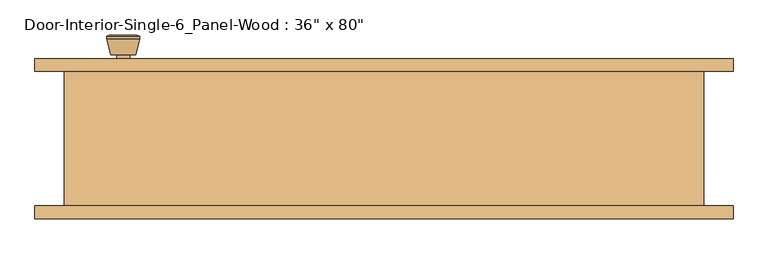
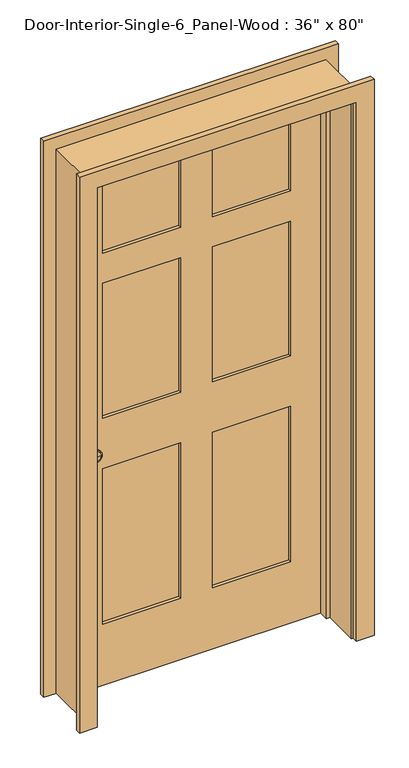
"""IFC4 building model written with IfcOpenShell, lengths in millimetres: door geometry."""

from ifc_helpers import new_model, si_unit, point, frame, frame_2d, origin, place, context, project, spatial, polyline, circle_curve, trimmed, segment, composite_curve, outline, extrude, faceted_brep, source, transform, mapped, element, save
from ifc_brep_helpers import plane_surface, cylinder_surface, revolved_surface, advanced_brep


def door_5dfbd760(model_context):
    return source(origin(), model_context, "Body", "SolidModel", [
        advanced_brep(
        [(-393.7, 57.5, 914.4), (-383.7, 57.5, 914.4), (-403.7, 57.5, 914.4), (-373.2241324, 8.5, 914.4), (-393.7, 8.5, 914.4), (-414.1758676, 8.5, 914.4), (-368.7, 10.3278681, 914.4), (-418.7, 10.3278681, 914.4), (-368.7, 13.7915463, 914.4), (-418.7, 13.7915463, 914.4), (-375.063764, 38.5, 914.4), (-412.336236, 38.5, 914.4), (-383.7, 38.5, 914.4), (-403.7, 38.5, 914.4)],
        [
            (0, 1),
            (1, 2, circle_curve(frame((-393.7, 57.5, 914.4), z_axis=(0.0, 1.0, 0.0), x_axis=(-1.0, 0.0, 0.0)), 10.0)),
            (2, 0),
            (2, 1, circle_curve(frame((-393.7, 57.5, 914.4), z_axis=(0.0, 1.0, 0.0), x_axis=(-1.0, 0.0, 0.0)), 10.0)),
            (3, 4),
            (4, 5),
            (5, 3, circle_curve(frame((-393.7, 8.5, 914.4), z_axis=(0.0, -1.0, 0.0), x_axis=(-1.0, 0.0, 0.0)), 20.4758676)),
            (3, 5, circle_curve(frame((-393.7, 8.5, 914.4), z_axis=(0.0, -1.0, 0.0), x_axis=(-1.0, 0.0, 0.0)), 20.4758676)),
            (6, 3),
            (5, 7),
            (7, 6, circle_curve(frame((-393.7, 10.3278681, 914.4), z_axis=(0.0, -1.0, 0.0), x_axis=(-1.0, 0.0, 0.0)), 25.0)),
            (6, 7, circle_curve(frame((-393.7, 10.3278681, 914.4), z_axis=(0.0, -1.0, 0.0), x_axis=(-1.0, 0.0, 0.0)), 25.0)),
            (8, 6),
            (7, 9),
            (9, 8, circle_curve(frame((-393.7, 13.7915463, 914.4), z_axis=(0.0, -1.0, 0.0), x_axis=(-1.0, 0.0, 0.0)), 25.0)),
            (8, 9, circle_curve(frame((-393.7, 13.7915463, 914.4), z_axis=(0.0, -1.0, 0.0), x_axis=(-1.0, 0.0, 0.0)), 25.0)),
            (10, 8),
            (9, 11),
            (11, 10, circle_curve(frame((-393.7, 38.5, 914.4), z_axis=(0.0, -1.0, 0.0), x_axis=(-1.0, 0.0, 0.0)), 18.636236)),
            (10, 11, circle_curve(frame((-393.7, 38.5, 914.4), z_axis=(0.0, -1.0, 0.0), x_axis=(-1.0, 0.0, 0.0)), 18.636236)),
            (12, 10),
            (11, 13),
            (13, 12, circle_curve(frame((-393.7, 38.5, 914.4), z_axis=(0.0, -1.0, 0.0), x_axis=(-1.0, 0.0, 0.0)), 10.0)),
            (12, 13, circle_curve(frame((-393.7, 38.5, 914.4), z_axis=(0.0, -1.0, 0.0), x_axis=(-1.0, 0.0, 0.0)), 10.0)),
            (1, 12),
            (13, 2),
        ],
        [
            plane_surface(frame((-393.7, 57.5, 914.4), z_axis=(0.0, 1.0, 0.0), x_axis=(-1.0, 0.0, 0.0))),
            plane_surface(frame((-393.7, 8.5, 914.4), z_axis=(0.0, -1.0, 0.0), x_axis=(-1.0, 0.0, 0.0))),
            revolved_surface(polyline([(-414.1758676, 8.5, 914.4), (-418.7, 10.3278681, 914.4)]), (-393.7, 57.5, 914.4), (0.0, 1.0, 0.0)),
            cylinder_surface(frame((-393.7, 57.5, 914.4), z_axis=(0.0, 1.0, 0.0), x_axis=(-1.0, 0.0, 0.0)), 25.0),
            revolved_surface(polyline([(-418.7, 13.7915463, 914.4), (-412.336236, 38.5, 914.4)]), (-393.7, 57.5, 914.4), (0.0, 1.0, 0.0)),
            plane_surface(frame((-393.7, 38.5, 914.4), z_axis=(0.0, 1.0, 0.0), x_axis=(-1.0, 0.0, 0.0))),
            cylinder_surface(frame((-393.7, 57.5, 914.4), z_axis=(0.0, 1.0, 0.0), x_axis=(-1.0, 0.0, 0.0)), 10.0),
        ],
        [
            (0, [[1, 2, 3]]),
            (0, [[-3, 4, -1]]),
            (1, [[5, 6, 7]]),
            (1, [[-6, -5, 8]]),
            (2, [[9, -7, 10, 11]]),
            (2, [[-10, -8, -9, 12]]),
            (3, [[13, -11, 14, 15]]),
            (3, [[-14, -12, -13, 16]]),
            (4, [[17, -15, 18, 19]]),
            (4, [[-18, -16, -17, 20]]),
            (5, [[21, -19, 22, 23]]),
            (5, [[-22, -20, -21, 24]]),
            (6, [[25, -23, 26, -2]]),
            (6, [[-26, -24, -25, -4]]),
        ],
    ),
        extrude(outline(composite_curve([segment(trimmed(circle_curve(frame_2d((914.4, -393.7)), 30.0), [point((914.4, -423.7))], [point((914.4, -363.7))], False, "CARTESIAN"), True, "CONTINUOUS"), segment(trimmed(circle_curve(frame_2d((914.4, -393.7)), 30.0), [point((914.4, -363.7))], [point((914.4, -423.7))], False, "CARTESIAN"), True, "CONTINUOUS")], self_intersect=False)), frame((0.0, 57.5, 0.0), z_axis=(0.0, 1.0, 0.0), x_axis=(0.0, 0.0, 1.0)), (0.0, 0.0, 1.0), 6.0),
        advanced_brep(
        [(-393.7, 104.425, 914.4), (-403.7, 104.425, 914.4), (-383.7, 104.425, 914.4), (-373.2241324, 153.425, 914.4), (-414.1758676, 153.425, 914.4), (-393.7, 153.425, 914.4), (-368.7, 151.5971319, 914.4), (-418.7, 151.5971319, 914.4), (-368.7, 148.1334537, 914.4), (-418.7, 148.1334537, 914.4), (-375.063764, 123.425, 914.4), (-412.336236, 123.425, 914.4), (-383.7, 123.425, 914.4), (-403.7, 123.425, 914.4)],
        [
            (0, 1),
            (1, 2, circle_curve(frame((-393.7, 104.425, 914.4), z_axis=(0.0, -1.0, 0.0), x_axis=(-1.0, 0.0, 0.0)), 10.0)),
            (2, 0),
            (2, 1, circle_curve(frame((-393.7, 104.425, 914.4), z_axis=(0.0, -1.0, 0.0), x_axis=(-1.0, 0.0, 0.0)), 10.0)),
            (3, 4, circle_curve(frame((-393.7, 153.425, 914.4), z_axis=(0.0, 1.0, 0.0), x_axis=(-1.0, 0.0, 0.0)), 20.4758676)),
            (4, 5),
            (5, 3),
            (4, 3, circle_curve(frame((-393.7, 153.425, 914.4), z_axis=(0.0, 1.0, 0.0), x_axis=(-1.0, 0.0, 0.0)), 20.4758676)),
            (6, 7, circle_curve(frame((-393.7, 151.5971319, 914.4), z_axis=(0.0, 1.0, 0.0), x_axis=(-1.0, 0.0, 0.0)), 25.0)),
            (7, 4),
            (3, 6),
            (7, 6, circle_curve(frame((-393.7, 151.5971319, 914.4), z_axis=(0.0, 1.0, 0.0), x_axis=(-1.0, 0.0, 0.0)), 25.0)),
            (8, 9, circle_curve(frame((-393.7, 148.1334537, 914.4), z_axis=(0.0, 1.0, 0.0), x_axis=(-1.0, 0.0, 0.0)), 25.0)),
            (9, 7),
            (6, 8),
            (9, 8, circle_curve(frame((-393.7, 148.1334537, 914.4), z_axis=(0.0, 1.0, 0.0), x_axis=(-1.0, 0.0, 0.0)), 25.0)),
            (10, 11, circle_curve(frame((-393.7, 123.425, 914.4), z_axis=(0.0, 1.0, 0.0), x_axis=(-1.0, 0.0, 0.0)), 18.636236)),
            (11, 9),
            (8, 10),
            (11, 10, circle_curve(frame((-393.7, 123.425, 914.4), z_axis=(0.0, 1.0, 0.0), x_axis=(-1.0, 0.0, 0.0)), 18.636236)),
            (12, 13, circle_curve(frame((-393.7, 123.425, 914.4), z_axis=(0.0, 1.0, 0.0), x_axis=(-1.0, 0.0, 0.0)), 10.0)),
            (13, 11),
            (10, 12),
            (13, 12, circle_curve(frame((-393.7, 123.425, 914.4), z_axis=(0.0, 1.0, 0.0), x_axis=(-1.0, 0.0, 0.0)), 10.0)),
            (1, 13),
            (12, 2),
        ],
        [
            plane_surface(frame((-393.7, 104.425, 914.4), z_axis=(0.0, -1.0, 0.0), x_axis=(-1.0, 0.0, 0.0))),
            plane_surface(frame((-393.7, 153.425, 914.4), z_axis=(0.0, 1.0, 0.0), x_axis=(-1.0, 0.0, 0.0))),
            revolved_surface(polyline([(-414.1758676, 153.425, 914.4), (-418.7, 151.5971319, 914.4)]), (-393.7, 104.425, 914.4), (0.0, -1.0, 0.0)),
            cylinder_surface(frame((-393.7, 104.425, 914.4), z_axis=(0.0, -1.0, 0.0), x_axis=(-1.0, 0.0, 0.0)), 25.0),
            revolved_surface(polyline([(-418.7, 148.1334537, 914.4), (-412.336236, 123.425, 914.4)]), (-393.7, 104.425, 914.4), (0.0, -1.0, 0.0)),
            plane_surface(frame((-393.7, 123.425, 914.4), z_axis=(0.0, -1.0, 0.0), x_axis=(-1.0, 0.0, 0.0))),
            cylinder_surface(frame((-393.7, 104.425, 914.4), z_axis=(0.0, -1.0, 0.0), x_axis=(-1.0, 0.0, 0.0)), 10.0),
        ],
        [
            (0, [[1, 2, 3]]),
            (0, [[-3, 4, -1]]),
            (1, [[5, 6, 7]]),
            (1, [[8, -7, -6]]),
            (2, [[9, 10, -5, 11]]),
            (2, [[12, -11, -8, -10]]),
            (3, [[13, 14, -9, 15]]),
            (3, [[16, -15, -12, -14]]),
            (4, [[17, 18, -13, 19]]),
            (4, [[20, -19, -16, -18]]),
            (5, [[21, 22, -17, 23]]),
            (5, [[24, -23, -20, -22]]),
            (6, [[-2, 25, -21, 26]]),
            (6, [[-4, -26, -24, -25]]),
        ],
    ),
        extrude(outline(composite_curve([segment(trimmed(circle_curve(frame_2d((914.4, -393.7)), 30.0), [point((914.4, -423.7))], [point((914.4, -363.7))], False, "CARTESIAN"), True, "CONTINUOUS"), segment(trimmed(circle_curve(frame_2d((914.4, -393.7)), 30.0), [point((914.4, -363.7))], [point((914.4, -423.7))], False, "CARTESIAN"), True, "CONTINUOUS")], self_intersect=False)), frame((0.0, 98.425, 0.0), z_axis=(0.0, 1.0, 0.0), x_axis=(0.0, 0.0, 1.0)), (0.0, 0.0, 1.0), 6.0),
        extrude(outline(polyline([(336.55, 75.1416667), (57.15, 75.1416667), (57.15, 86.7833333), (336.55, 86.7833333), (336.55, 75.1416667)])), frame((0.0, 0.0, 1633.5375), z_axis=(0.0, 0.0, 1.0), x_axis=(1.0, 0.0, 0.0)), (0.0, 0.0, 1.0), 279.4),
        extrude(outline(polyline([(336.55, 75.1416667), (57.15, 75.1416667), (57.15, 86.7833333), (336.55, 86.7833333), (336.55, 75.1416667)])), frame((0.0, 0.0, 1009.65), z_axis=(0.0, 0.0, 1.0), x_axis=(1.0, 0.0, 0.0)), (0.0, 0.0, 1.0), 509.5875),
        extrude(outline(polyline([(-57.15, 75.1416667), (-336.55, 75.1416667), (-336.55, 86.7833333), (-57.15, 86.7833333), (-57.15, 75.1416667)])), frame((0.0, 0.0, 1009.65), z_axis=(0.0, 0.0, 1.0), x_axis=(1.0, 0.0, 0.0)), (0.0, 0.0, 1.0), 509.5875),
        extrude(outline(polyline([(-57.15, 75.1416667), (-336.55, 75.1416667), (-336.55, 86.7833333), (-57.15, 86.7833333), (-57.15, 75.1416667)])), frame((0.0, 0.0, 1633.5375), z_axis=(0.0, 0.0, 1.0), x_axis=(1.0, 0.0, 0.0)), (0.0, 0.0, 1.0), 279.4),
        extrude(outline(polyline([(336.55, 75.1416667), (57.15, 75.1416667), (57.15, 86.7833333), (336.55, 86.7833333), (336.55, 75.1416667)])), frame((0.0, 0.0, 231.775), z_axis=(0.0, 0.0, 1.0), x_axis=(1.0, 0.0, 0.0)), (0.0, 0.0, 1.0), 587.375),
        extrude(outline(polyline([(-57.15, 75.1416667), (-336.55, 75.1416667), (-336.55, 86.7833333), (-57.15, 86.7833333), (-57.15, 75.1416667)])), frame((0.0, 0.0, 231.775), z_axis=(0.0, 0.0, 1.0), x_axis=(1.0, 0.0, 0.0)), (0.0, 0.0, 1.0), 587.375),
        extrude(outline(polyline([(2032.0, -457.2), (0.0, -457.2), (0.0, 457.2), (2032.0, 457.2), (2032.0, -457.2)]), holes=[polyline([(1912.9375, 57.15), (1912.9375, 336.55), (1633.5375, 336.55), (1633.5375, 57.15), (1912.9375, 57.15)]), polyline([(1519.2375, 336.55), (1009.65, 336.55), (1009.65, 57.15), (1519.2375, 57.15), (1519.2375, 336.55)]), polyline([(1009.65, -57.15), (1009.65, -336.55), (1519.2375, -336.55), (1519.2375, -57.15), (1009.65, -57.15)]), polyline([(1633.5375, -336.55), (1912.9375, -336.55), (1912.9375, -57.15), (1633.5375, -57.15), (1633.5375, -336.55)]), polyline([(819.15, 57.15), (819.15, 336.55), (231.775, 336.55), (231.775, 57.15), (819.15, 57.15)]), polyline([(231.775, -57.15), (231.775, -336.55), (819.15, -336.55), (819.15, -57.15), (231.775, -57.15)])]), frame((0.0, 63.5, 0.0), z_axis=(0.0, 1.0, 0.0), x_axis=(0.0, 0.0, 1.0)), (0.0, 0.0, 1.0), 34.925),
        faceted_brep([(482.6, 98.425, 0.0), (482.6, -104.775, 0.0), (457.2, -104.775, 0.0), (457.2, 28.575, 0.0), (444.5, 28.575, 0.0), (444.5, 63.5, 0.0), (457.2, 63.5, 0.0), (457.2, 98.425, 0.0), (482.6, 98.425, 2057.4), (482.6, -104.775, 2057.4), (-482.6, -104.775, 2057.4), (-482.6, -104.775, 0.0), (-457.2, -104.775, 0.0), (-457.2, -104.775, 2032.0), (457.2, -104.775, 2032.0), (457.2, 28.575, 2032.0), (-457.2, 28.575, 2032.0), (-457.2, 28.575, 0.0), (-444.5, 28.575, 0.0), (-444.5, 28.575, 2019.3), (444.5, 28.575, 2019.3), (444.5, 63.5, 2019.3), (-444.5, 63.5, 2019.3), (-444.5, 63.5, 0.0), (-457.2, 63.5, 0.0), (-457.2, 63.5, 2032.0), (457.2, 63.5, 2032.0), (457.2, 98.425, 2032.0), (-457.2, 98.425, 2032.0), (-457.2, 98.425, 0.0), (-482.6, 98.425, 0.0), (-482.6, 98.425, 2057.4)], [[[0, 1, 2, 3, 4, 5, 6, 7]], [[1, 0, 8, 9]], [[2, 1, 9, 10, 11, 12, 13, 14]], [[3, 2, 14, 15]], [[4, 3, 15, 16, 17, 18, 19, 20]], [[5, 4, 20, 21]], [[6, 5, 21, 22, 23, 24, 25, 26]], [[7, 6, 26, 27]], [[0, 7, 27, 28, 29, 30, 31, 8]], [[9, 8, 31, 10]], [[15, 14, 13, 16]], [[21, 20, 19, 22]], [[27, 26, 25, 28]], [[30, 29, 24, 23, 18, 17, 12, 11]], [[10, 31, 30, 11]], [[16, 13, 12, 17]], [[22, 19, 18, 23]], [[28, 25, 24, 29]]]),
        extrude(outline(polyline([(0.0, 463.55), (0.0, 527.05), (2101.85, 527.05), (2101.85, -527.05), (0.0, -527.05), (0.0, -463.55), (2038.35, -463.55), (2038.35, 463.55), (0.0, 463.55)])), frame((0.0, -123.825, 0.0), z_axis=(0.0, 1.0, 0.0), x_axis=(0.0, 0.0, 1.0)), (0.0, 0.0, 1.0), 19.05),
        extrude(outline(polyline([(0.0, 463.55), (0.0, 527.05), (2101.85, 527.05), (2101.85, -527.05), (0.0, -527.05), (0.0, -463.55), (2038.35, -463.55), (2038.35, 463.55), (0.0, 463.55)])), frame((0.0, 98.425, 0.0), z_axis=(0.0, 1.0, 0.0), x_axis=(0.0, 0.0, 1.0)), (0.0, 0.0, 1.0), 19.05),
    ])


if __name__ == "__main__":
    model = new_model("IFC4")
    model_context = context("Model", 3, world=origin())
    ifc_project = project(units=[si_unit("LENGTHUNIT", "METRE", prefix="MILLI")], contexts=[model_context])
    site = spatial("IfcSite", under=ifc_project)
    building = spatial("IfcBuilding", under=site)
    placement = place(None, origin())
    door_shape = door_5dfbd760(model_context)
    element("IfcDoor", 1, ObjectType="Door-Interior-Single-6_Panel-Wood : 36\" x 80\"", at=placement, inside=building, context=model_context, shape_type="MappedRepresentation", body=[
        mapped(door_shape, transform((0.0, 0.0, 0.0), x_axis=(1.0, 0.0, 0.0), y_axis=(0.0, 1.0, 0.0), z_axis=(0.0, 0.0, 1.0))),
    ])
    save(model, "model.ifc")

# Revit data of these elements
# Type "Door-Interior-Single-6_Panel-Wood : 36\" x 80\""
#   Type Mark = "9"
#   Assembly Code = "C1020300"
#   Analytic Construction = "Wooden"
#   Top Rail = 0' - 4 11/16"
#   Top Panel = 0' - 11"
#   Thickness = 0' - 1 3/8"
#   Thermal Resistance (R) = 2.5876 (h·ft²·°F)/BTU
#   Swing Angle [instance default] = 90.00°
#   Stiles = 0' - 4 3/4"
#   Rough Width = 3' - 2"
#   Rough Height = 6' - 9"
#   Mullion = 0' - 4 1/2"
#   Lock Rail = 0' - 7 1/2"
#   Intermediate Rail = 0' - 4 1/2"
#   Height = 6' - 8"
#   Width = 3' - 0"
#   Heat Transfer Coefficient (U) = 0.3865 BTU/(h·ft²·°F)
#   Bottom Rail = 0' - 9 1/8"
#   Trim Material = Cherry
#   Panel Material = Cherry
#   Frame Material = Cherry
#   Door Handle Material = Aluminum
#   Visual Light Transmittance = 0
#   Solar Heat Gain Coefficient = 0
#   Wall Closure = (empty or 0)
#   Function = (empty or 0)
# Element 1 (IfcDoor, "Door-Interior-Single-6_Panel-Wood : 36\" x 80\"")
#   Materials on its faces: "Cherry", "Aluminum"
# Materials
#   "Cherry": class "Wood", colour RGB 226 177 128, transparency 0, Description = "Prunus Serotina", Cost = 0
#   "Aluminum": class "Metal", colour RGB 247 247 247, transparency 0, Description = "Aluminum 6061", Cost = 0
